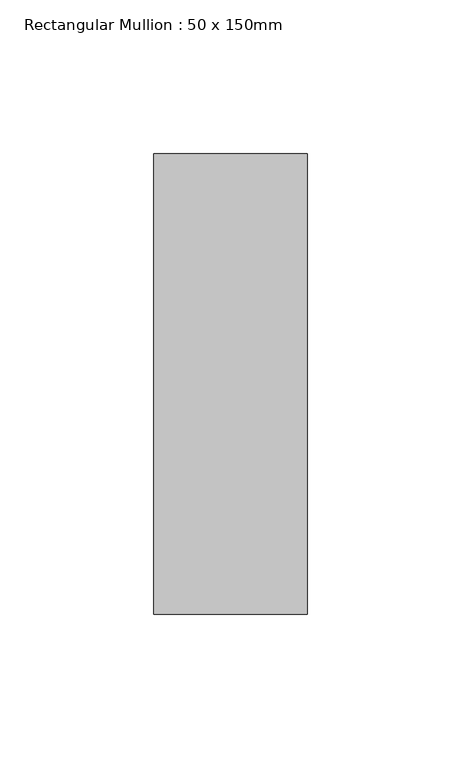
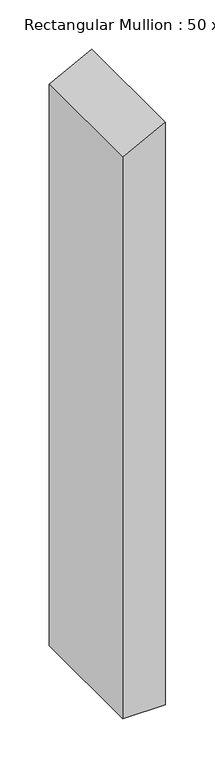
"""IFC4 building model written with IfcOpenShell, lengths in millimetres: member geometry, Rectangular Mullion : 50 x 150mm."""

from ifc_helpers import new_model, si_unit, frame, origin, place, context, project, spatial, polyline, outline, extrude, source, transform, mapped, element, save


def rectangular_mullion_50_x_150mm_405b5ff6(model_context):
    return source(origin(), model_context, "Body", "SweptSolid", [
        extrude(outline(polyline([(0.0, 0.0), (-26.0283525, -50.0), (-723.4218706, -50.0), (-723.4218706, 0.0), (0.0, 0.0)])), frame((0.0, -75.0, 0.0), z_axis=(0.0, 1.0, 0.0), x_axis=(0.0, 0.0, 1.0)), (0.0, 0.0, 1.0), 150.0),
    ])


if __name__ == "__main__":
    model = new_model("IFC4")
    model_context = context("Model", 3, world=origin())
    ifc_project = project(units=[si_unit("LENGTHUNIT", "METRE", prefix="MILLI")], contexts=[model_context])
    site = spatial("IfcSite", under=ifc_project)
    building = spatial("IfcBuilding", under=site)
    placement = place(None, origin())
    rectangular_mullion_50_x_150mm_shape = rectangular_mullion_50_x_150mm_405b5ff6(model_context)
    element("IfcMember", 1, ObjectType="Rectangular Mullion : 50 x 150mm", at=placement, inside=building, context=model_context, shape_type="MappedRepresentation", body=[
        mapped(rectangular_mullion_50_x_150mm_shape, transform((0.0, 0.0, 0.0), x_axis=(1.0, 0.0, 0.0), y_axis=(0.0, 1.0, 0.0), z_axis=(0.0, 0.0, 1.0))),
    ])
    save(model, "model.ifc")

# Revit data of these elements
# Type "Rectangular Mullion : 50 x 150mm"
#   built-in parameter 1007304 = 0.492126 (stored number, unit not read)
#   built-in parameter 1007301 = 0.082021 (stored number, unit not read)
#   built-in parameter 1007300 = 0.082021 (stored number, unit not read)
# Element 1 (IfcMember, "Rectangular Mullion : 50 x 150mm")
#   Materials on its faces: "Aluminium"
# Materials
#   "Aluminium": class "Metal", colour RGB 247 247 247, transparency 0, Description = "Aluminium 6061", Cost = 0
